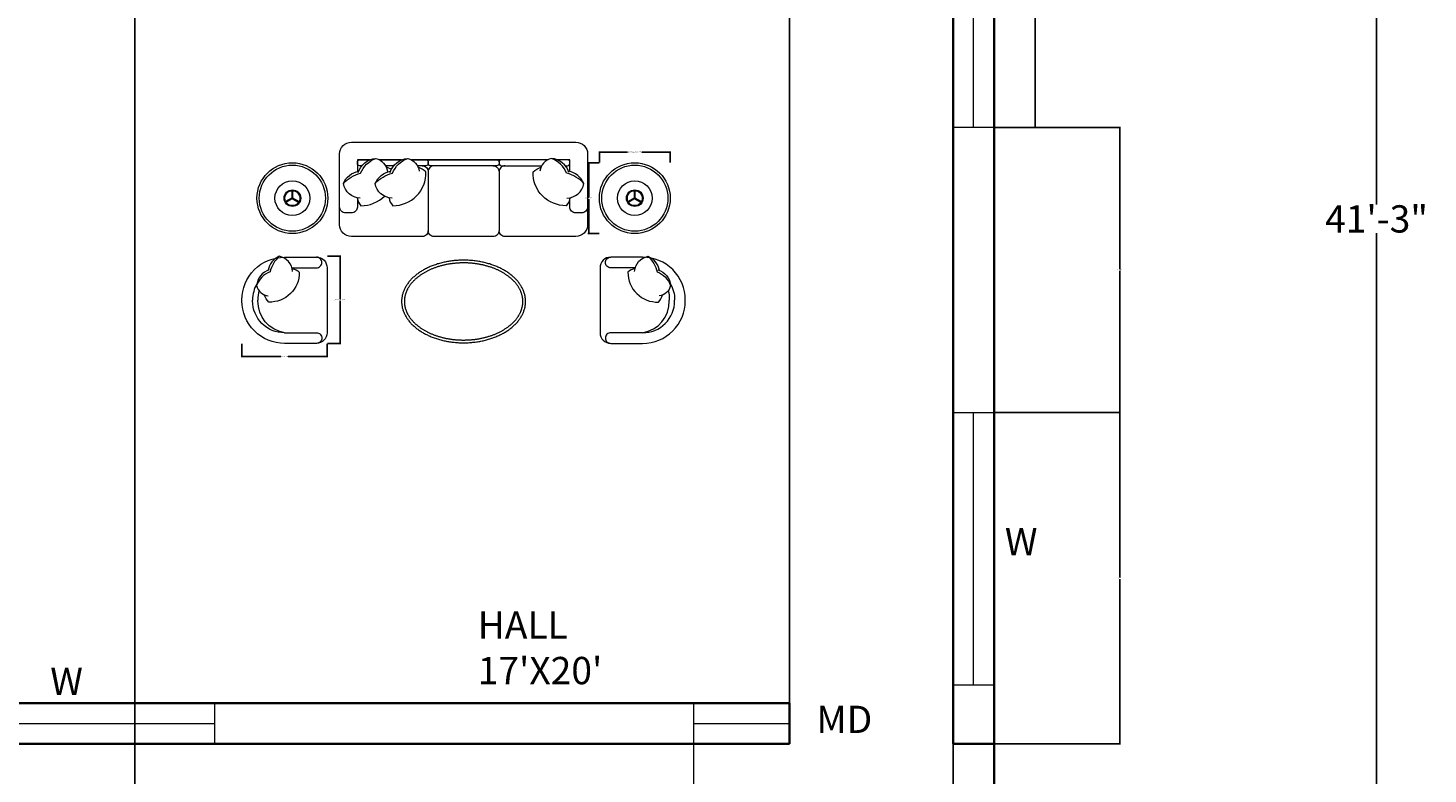
# Model space of a CAD drawing. Units: inches. Extents: x -4347 to -3836, y 955 to 1521.
# Tile 8 of 11: x -4144 to -3836, y 1120 to 1284. Entities that reach past the tile are written whole.
import ezdxf

# ---------------------------------------------------------------- set-up
doc = ezdxf.new("R2010")
doc.units = ezdxf.units.IN
doc.header["$MEASUREMENT"] = 0
for name, color, linetype, lineweight in [('A-ANNO-DIMS', 2, 'Continuous', 18), ('A-ANNO-TEXT', 7, 'Continuous', 18), ('A-AREA-IDEN', 7, 'Continuous', 18), ('A-FLOR-STRS', 7, 'Continuous', 18), ('A-FURN', 8, 'Continuous', 13), ('A-GLAZ', 4, 'Continuous', 18), ('A-WALL', 7, 'Continuous', 35)]:
    doc.layers.add(name, color=color, linetype=linetype, lineweight=lineweight)
doc.styles.get("Standard").update_dxf_attribs({"font": 'arial.ttf'})
doc.dimstyles.get("Standard").update_dxf_attribs({"dimtxt": 0.18, "dimasz": 0.18, "dimexe": 0.18, "dimexo": 0.0625, "dimgap": 0.09, "dimtad": 0, "dimtih": 1, "dimtoh": 1, "dimdec": 0, "dimzin": 0, "dimdsep": 46, "dimlunit": 3, "dimtxsty": 'Standard', "dimcen": 0.09, "dimadec": 0, "dimazin": 0, "dimtfac": 1, "dimtdec": 0, "dimtofl": 0, "dimtmove": 0, "dimatfit": 3, "dimfxl": 1, "dimtolj": 1, "dimtzin": 0, "dimarcsym": 0})

# ---------------------------------------------------------------- blocks, each defined once
blk = doc.blocks.new('*D2')
at = {"layer": 'A-ANNO-DIMS', "color": 0, "lineweight": -2, "transparency": 16777216}
for p, q in [((-3931.52, 1489.79), (-3847.29, 1489.79)), ((-3847.47, 1489.61), (-3847.47, 1245.44)), ((-3847.47, 994.97), (-3847.47, 1239.13)), ((-3931.52, 994.79), (-3847.29, 994.79))]:
    blk.add_line(p, q, dxfattribs=at)
at = {"layer": 'A-ANNO-DIMS', "color": 0, "transparency": 16777216}
for points in [[(-3847.5, 1489.61), (-3847.44, 1489.61), (-3847.47, 1489.79)], [(-3847.5, 994.97), (-3847.44, 994.97), (-3847.47, 994.79)]]:
    blk.add_solid(points, dxfattribs=at)
at = {"layer": 'Defpoints', "color": 0, "transparency": 16777216}
for p in [(-3931.58, 1489.79), (-3931.58, 994.79), (-3847.47, 994.79)]:
    blk.add_point(p, dxfattribs=at)
at = {"layer": 'A-ANNO-DIMS', "color": 0, "transparency": 16777216, "insert": (-3847.47, 1242.29), "char_height": 6, "attachment_point": 5}
blk.add_mtext('\\A1;41\'-3"', dxfattribs=at)
blk = doc.blocks.new('ARMCHAIR')
at = {"ltscale": 0.03}
blk.add_lwpolyline([(18.73, 9.48), (18.73, 2.34, -0.414214), (16.39, 0), (9.37, 0, -0.414214), (0, 9.37), (0, 9.48), (0, 9.6, -0.414214), (9.37, 18.97), (16.39, 18.97, -0.414214), (18.73, 16.62), (18.73, 9.48)], format="xyb", dxfattribs=at)
for points in [[(8.18, 19.16, 0.14773), (6.17, 15.73, 0.213343), (3.22, 12.72, 0.178662)], [(11.13, 15.8, 0.356772), (8.18, 19.16, 0.249542), (5.75, 16.12, -9.61688)], [(11.01, 16.62), (16.39, 16.62, 0.414214), (17.56, 17.79), (17.56, 17.79, 0.414214), (16.39, 18.97)], [(6.01, 16.21, 0.306663), (3.22, 12.72, 0.30633), (5.77, 10.43, -0.872847)], [(11.06, 16.39, -0.165541), (12.61, 15.67, -0.425989), (5.9, 9.09, -0.121523), (4.98, 10.65, 7.115464)], [(3.27, 13.09, 0.130591), (2.34, 9.6), (2.34, 9.48)], [(9.37, 2.34, -0.414214), (2.34, 9.37), (2.34, 9.48)], [(3.76, 11.6, 0.072384), (3.51, 9.6), (3.51, 9.48)], [(9.37, 2.34, -0.372719), (3.51, 9.37), (3.51, 9.48)], [(9.37, 2.34), (16.39, 2.34, -0.414214), (17.56, 1.17), (17.56, 1.17, -0.414214), (16.39, 0)]]:
    blk.add_lwpolyline(points, format="xyb")
blk = doc.blocks.new('END-TABLE-ROUND')
at = {"ltscale": 0.03}
for p, q in [((7.71, 7.79), (7.71, 9.62)), ((7.87, 7.79), (7.87, 9.62)), ((7.75, 7.86), (6.16, 6.95)), ((7.83, 7.72), (6.25, 6.8)), ((7.75, 7.72), (9.34, 6.8)), ((7.83, 7.86), (9.42, 6.95))]:
    blk.add_line(p, q, dxfattribs=at)
for radius in [7.79, 3.83, 1.83, 1.64]:
    blk.add_circle((7.79, 7.79), radius, dxfattribs=at)
blk.add_circle((7.79, 7.79), 7.27)
blk = doc.blocks.new('GLAZ-60IN')
for p, q in [((0, 9), (60, 9)), ((0, 0), (0, 9)), ((60, 9), (60, 0)), ((0, 4.5), (60, 4.5)), ((60, 0), (0, 0))]:
    blk.add_line(p, q)
blk = doc.blocks.new('*D20')
at = {"layer": 'A-ANNO-DIMS', "color": 0, "lineweight": -2, "transparency": 16777216}
for p, q in [((-4078.22, 1234.06), (-4075.23, 1234.06)), ((-4075.41, 1233.88), (-4075.41, 1224.66)), ((-4075.41, 1215.08), (-4075.41, 1224.3)), ((-4078.22, 1214.9), (-4075.23, 1214.9))]:
    blk.add_line(p, q, dxfattribs=at)
at = {"layer": 'A-ANNO-DIMS', "color": 0, "transparency": 16777216}
for points in [[(-4075.44, 1233.88), (-4075.38, 1233.88), (-4075.41, 1234.06)], [(-4075.44, 1215.08), (-4075.38, 1215.08), (-4075.41, 1214.9)]]:
    blk.add_solid(points, dxfattribs=at)
at = {"layer": 'Defpoints', "color": 0, "transparency": 16777216}
for p in [(-4078.28, 1234.06), (-4075.41, 1234.06), (-4078.28, 1214.9)]:
    blk.add_point(p, dxfattribs=at)
at = {"layer": 'A-ANNO-DIMS', "color": 0, "transparency": 16777216, "insert": (-4075.41, 1224.48), "char_height": 0.18, "attachment_point": 5}
blk.add_mtext('\\A1;ARMCHAIR 1\'-7" TYP.', dxfattribs=at)
blk = doc.blocks.new('*D21')
at = {"layer": 'A-ANNO-DIMS', "color": 0, "lineweight": -2, "transparency": 16777216}
for p, q in [((-4097.01, 1214.84), (-4097.01, 1211.85)), ((-4078.28, 1214.84), (-4078.28, 1211.85)), ((-4096.83, 1212.03), (-4088.49, 1212.03)), ((-4078.46, 1212.03), (-4086.81, 1212.03))]:
    blk.add_line(p, q, dxfattribs=at)
at = {"layer": 'A-ANNO-DIMS', "color": 0, "transparency": 16777216}
for points in [[(-4096.83, 1212.06), (-4096.83, 1212), (-4097.01, 1212.03)], [(-4078.46, 1212.06), (-4078.46, 1212), (-4078.28, 1212.03)]]:
    blk.add_solid(points, dxfattribs=at)
at = {"layer": 'Defpoints', "color": 0, "transparency": 16777216}
for p in [(-4097.01, 1214.9), (-4078.28, 1214.9), (-4078.28, 1212.03)]:
    blk.add_point(p, dxfattribs=at)
at = {"layer": 'A-ANNO-DIMS', "color": 0, "transparency": 16777216, "insert": (-4087.65, 1212.03), "char_height": 0.18, "attachment_point": 5}
blk.add_mtext('\\A1;1\'-6 1/2" TYP.', dxfattribs=at)
blk = doc.blocks.new('*D22')
at = {"layer": 'A-ANNO-DIMS', "color": 0, "lineweight": -2, "transparency": 16777216}
for p, q in [((-4018.4, 1254.7), (-4018.4, 1257.15)), ((-4018.22, 1256.97), (-4012.18, 1256.97)), ((-4003, 1256.97), (-4009.03, 1256.97)), ((-4002.82, 1254.7), (-4002.82, 1257.15))]:
    blk.add_line(p, q, dxfattribs=at)
at = {"layer": 'A-ANNO-DIMS', "color": 0, "transparency": 16777216}
for points in [[(-4018.22, 1257), (-4018.22, 1256.94), (-4018.4, 1256.97)], [(-4003, 1257), (-4003, 1256.94), (-4002.82, 1256.97)]]:
    blk.add_solid(points, dxfattribs=at)
at = {"layer": 'Defpoints', "color": 0, "transparency": 16777216}
for p in [(-4002.82, 1256.97), (-4018.4, 1254.64), (-4002.82, 1254.64)]:
    blk.add_point(p, dxfattribs=at)
at = {"layer": 'A-ANNO-DIMS', "color": 0, "transparency": 16777216, "insert": (-4010.61, 1256.97), "char_height": 0.18, "attachment_point": 5}
blk.add_mtext('\\A1;END TABLE 1\'-3 1/2" TYP.', dxfattribs=at)
blk = doc.blocks.new('*D23')
at = {"layer": 'A-ANNO-DIMS', "color": 0, "lineweight": -2, "transparency": 16777216}
for p, q in [((-4018.46, 1254.64), (-4020.91, 1254.64)), ((-4020.73, 1254.46), (-4020.73, 1247.03)), ((-4020.73, 1239.24), (-4020.73, 1246.66)), ((-4018.46, 1239.06), (-4020.91, 1239.06))]:
    blk.add_line(p, q, dxfattribs=at)
at = {"layer": 'A-ANNO-DIMS', "color": 0, "transparency": 16777216}
for points in [[(-4020.76, 1254.46), (-4020.7, 1254.46), (-4020.73, 1254.64)], [(-4020.76, 1239.24), (-4020.7, 1239.24), (-4020.73, 1239.06)]]:
    blk.add_solid(points, dxfattribs=at)
at = {"layer": 'Defpoints', "color": 0, "transparency": 16777216}
for p in [(-4020.73, 1254.64), (-4018.4, 1254.64), (-4018.4, 1239.06)]:
    blk.add_point(p, dxfattribs=at)
at = {"layer": 'A-ANNO-DIMS', "color": 0, "transparency": 16777216, "insert": (-4020.73, 1246.85), "char_height": 0.18, "attachment_point": 5}
blk.add_mtext('\\A1;1\'-3 1/2" TYP.', dxfattribs=at)
blk = doc.blocks.new('*D28')
at = {"layer": 'A-ANNO-DIMS', "color": 0, "lineweight": -2, "transparency": 16777216}
for p, q in [((-3931.52, 1322.43), (-3922.4, 1322.43)), ((-3922.58, 1322.25), (-3922.58, 1292.61)), ((-3922.58, 1262.61), (-3922.58, 1292.25)), ((-3931.52, 1262.43), (-3922.4, 1262.43))]:
    blk.add_line(p, q, dxfattribs=at)
at = {"layer": 'A-ANNO-DIMS', "color": 0, "transparency": 16777216}
for points in [[(-3922.61, 1322.25), (-3922.55, 1322.25), (-3922.58, 1322.43)], [(-3922.61, 1262.61), (-3922.55, 1262.61), (-3922.58, 1262.43)]]:
    blk.add_solid(points, dxfattribs=at)
at = {"layer": 'Defpoints', "color": 0, "transparency": 16777216}
for p in [(-3931.58, 1322.43), (-3922.58, 1322.43), (-3931.58, 1262.43)]:
    blk.add_point(p, dxfattribs=at)
at = {"layer": 'A-ANNO-DIMS', "color": 0, "transparency": 16777216, "insert": (-3922.58, 1292.43), "char_height": 0.18, "attachment_point": 5}
blk.add_mtext('\\A1;GLAZING 5\'-0" TYP.', dxfattribs=at)
blk = doc.blocks.new('*D44')
at = {"layer": 'A-ANNO-DIMS', "color": 0, "lineweight": -2, "transparency": 16777216}
for p, q in [((-3931.52, 1199.71), (-3903.75, 1199.71)), ((-3903.93, 1199.53), (-3903.93, 1163.43)), ((-3903.93, 1126.97), (-3903.93, 1163.07)), ((-3931.52, 1126.79), (-3903.75, 1126.79))]:
    blk.add_line(p, q, dxfattribs=at)
at = {"layer": 'A-ANNO-DIMS', "color": 0, "transparency": 16777216}
for points in [[(-3903.96, 1199.53), (-3903.9, 1199.53), (-3903.93, 1199.71)], [(-3903.96, 1126.97), (-3903.9, 1126.97), (-3903.93, 1126.79)]]:
    blk.add_solid(points, dxfattribs=at)
at = {"layer": 'Defpoints', "color": 0, "transparency": 16777216}
for p in [(-3931.58, 1199.71), (-3903.93, 1199.71), (-3931.58, 1126.79)]:
    blk.add_point(p, dxfattribs=at)
at = {"layer": 'A-ANNO-DIMS', "color": 0, "transparency": 16777216, "insert": (-3903.93, 1163.25), "char_height": 0.18, "attachment_point": 5}
blk.add_mtext('\\A1;6\'-1"', dxfattribs=at)
blk = doc.blocks.new('*D45')
at = {"layer": 'A-ANNO-DIMS', "color": 0, "lineweight": -2, "transparency": 16777216}
for p, q in [((-3931.52, 1262.43), (-3903.75, 1262.43)), ((-3903.93, 1262.25), (-3903.93, 1231.25)), ((-3903.93, 1199.89), (-3903.93, 1230.89)), ((-3931.52, 1199.71), (-3903.75, 1199.71))]:
    blk.add_line(p, q, dxfattribs=at)
at = {"layer": 'A-ANNO-DIMS', "color": 0, "transparency": 16777216}
for points in [[(-3903.96, 1262.25), (-3903.9, 1262.25), (-3903.93, 1262.43)], [(-3903.96, 1199.89), (-3903.9, 1199.89), (-3903.93, 1199.71)]]:
    blk.add_solid(points, dxfattribs=at)
at = {"layer": 'Defpoints', "color": 0, "transparency": 16777216}
for p in [(-3931.58, 1262.43), (-3903.93, 1262.43), (-3931.58, 1199.71)]:
    blk.add_point(p, dxfattribs=at)
at = {"layer": 'A-ANNO-DIMS', "color": 0, "transparency": 16777216, "insert": (-3903.93, 1231.07), "char_height": 0.18, "attachment_point": 5}
blk.add_mtext('\\A1;5\'-2 1/2"', dxfattribs=at)
blk = doc.blocks.new('*D47')
at = {"layer": 'A-ANNO-DIMS', "color": 0, "lineweight": -2, "transparency": 16777216}
for p, q in [((-4120.58, 1288.73), (-4120.58, 966.96)), ((-3940.58, 1288.73), (-3940.58, 966.96)), ((-4120.4, 967.14), (-4030.97, 967.14)), ((-3940.76, 967.14), (-4030.19, 967.14))]:
    blk.add_line(p, q, dxfattribs=at)
at = {"layer": 'A-ANNO-DIMS', "color": 0, "transparency": 16777216}
for points in [[(-4120.4, 967.17), (-4120.4, 967.11), (-4120.58, 967.14)], [(-3940.76, 967.17), (-3940.76, 967.11), (-3940.58, 967.14)]]:
    blk.add_solid(points, dxfattribs=at)
at = {"layer": 'Defpoints', "color": 0, "transparency": 16777216}
for p in [(-4120.58, 1288.79), (-3940.58, 1288.79), (-3940.58, 967.14)]:
    blk.add_point(p, dxfattribs=at)
at = {"layer": 'A-ANNO-DIMS', "color": 0, "transparency": 16777216, "insert": (-4030.58, 967.14), "char_height": 0.18, "attachment_point": 5}
blk.add_mtext('\\A1;15\'-0"', dxfattribs=at)
blk = doc.blocks.new('*D53')
at = {"layer": 'A-ANNO-DIMS', "color": 0, "lineweight": -2, "transparency": 16777216}
for p, q in [((-3976.58, 1135.85), (-3976.58, 1517.62)), ((-3976.4, 1517.44), (-3958.91, 1517.44)), ((-3940.76, 1517.44), (-3958.25, 1517.44)), ((-3940.58, 1135.85), (-3940.58, 1517.62))]:
    blk.add_line(p, q, dxfattribs=at)
at = {"layer": 'A-ANNO-DIMS', "color": 0, "transparency": 16777216}
for points in [[(-3976.4, 1517.47), (-3976.4, 1517.41), (-3976.58, 1517.44)], [(-3940.76, 1517.47), (-3940.76, 1517.41), (-3940.58, 1517.44)]]:
    blk.add_solid(points, dxfattribs=at)
at = {"layer": 'Defpoints', "color": 0, "transparency": 16777216}
for p in [(-3940.58, 1517.44), (-3976.58, 1135.79), (-3940.58, 1135.79)]:
    blk.add_point(p, dxfattribs=at)
at = {"layer": 'A-ANNO-DIMS', "color": 0, "transparency": 16777216, "insert": (-3958.58, 1517.44), "char_height": 0.18, "attachment_point": 5}
blk.add_mtext('\\A1;3\'-0"', dxfattribs=at)
blk = doc.blocks.new('*D54')
at = {"layer": 'A-ANNO-DIMS', "color": 0, "lineweight": -2, "transparency": 16777216}
for p, q in [((-3997.76, 1126.79), (-4346.41, 1126.79)), ((-4346.23, 1126.61), (-4346.23, 1111.97)), ((-4346.23, 1096.97), (-4346.23, 1111.61)), ((-3997.76, 1096.79), (-4346.41, 1096.79))]:
    blk.add_line(p, q, dxfattribs=at)
at = {"layer": 'A-ANNO-DIMS', "color": 0, "transparency": 16777216}
for points in [[(-4346.26, 1126.61), (-4346.2, 1126.61), (-4346.23, 1126.79)], [(-4346.26, 1096.97), (-4346.2, 1096.97), (-4346.23, 1096.79)]]:
    blk.add_solid(points, dxfattribs=at)
at = {"layer": 'Defpoints', "color": 0, "transparency": 16777216}
for p in [(-4346.23, 1126.79), (-3997.69, 1126.79), (-3997.69, 1096.79)]:
    blk.add_point(p, dxfattribs=at)
at = {"layer": 'A-ANNO-DIMS', "color": 0, "transparency": 16777216, "insert": (-4346.23, 1111.79), "char_height": 0.18, "attachment_point": 5}
blk.add_mtext('\\A1;2\'-6"', dxfattribs=at)

msp = doc.modelspace()

# ---------------------------------------------------------------- linework, layer by layer
at = {"layer": 'A-FLOR-STRS'}
msp.add_line((-3997.69, 1126.79), (-3997.69, 1116.79), dxfattribs=at)
at = {"layer": 'A-FURN', "ltscale": 0.03}
msp.add_lwpolyline([(-4020.99, 1241, -0.414214), (-4023.59, 1238.41), (-4039.17, 1238.41, -0.414214), (-4040.47, 1239.7, -0.414214), (-4041.77, 1238.41), (-4054.75, 1238.41, -0.414214), (-4056.05, 1239.7, -0.414214), (-4057.35, 1238.41), (-4072.93, 1238.41, -0.414214), (-4075.53, 1241), (-4075.53, 1256.58, -0.414214), (-4072.93, 1259.18), (-4023.59, 1259.18, -0.414214), (-4020.99, 1256.58)], format="xyb", close=True, dxfattribs=at)
at = {"layer": 'A-FURN'}
for points in [[(-4074.7, 1250.1, -0.14773), (-4070.91, 1252.34, -0.213343), (-4067.56, 1255.61, -0.178662)], [(-4068.9, 1255.29), (-4071.63, 1255.29), (-4071.63, 1252.73, -0.414214)], [(-4070.64, 1253.99), (-4071.11, 1253.99, -0.414214), (-4071.63, 1254.51), (-4071.63, 1254.77, -0.414214), (-4071.11, 1255.29)], [(-4071.43, 1252.51, -0.306663), (-4067.56, 1255.61, -0.30633), (-4065.03, 1252.78, 0.872847)], [(-4071.11, 1255.29), (-4068.9, 1255.29, -0.414214)], [(-4067.71, 1250.1, -0.14773), (-4063.91, 1252.34, -0.213343), (-4060.56, 1255.61, -0.178662)], [(-4066.74, 1255.29), (-4061.91, 1255.29, -0.414214)], [(-4063.65, 1253.99), (-4065.43, 1253.99, -0.414214)], [(-4064.18, 1253.15, 0.071865), (-4065.27, 1253.66, -7.115464)], [(-4064.64, 1246.91, 0.165541), (-4063.84, 1245.2, 0.425989), (-4056.55, 1252.63, 0.121523), (-4058.28, 1253.66, -7.115464)], [(-4064.44, 1252.51, -0.306663), (-4060.56, 1255.61, -0.30633), (-4058.03, 1252.78, 0.872847)], [(-4059.75, 1255.29), (-4056.57, 1255.29, -0.414214), (-4056.05, 1254.77), (-4056.05, 1254.51, -0.414214), (-4056.57, 1253.99), (-4058.44, 1253.99, -0.414214)], [(-4057.35, 1253.99, -0.414214), (-4056.05, 1252.69), (-4056.05, 1239.7, -0.414214)], [(-4054.75, 1253.99, 0.414214), (-4056.05, 1252.69)], [(-4041.77, 1253.99, -0.414214), (-4040.47, 1252.69)], [(-4029.78, 1255.29), (-4039.95, 1255.29, 0.414214), (-4040.47, 1254.77), (-4040.47, 1254.51, 0.414214), (-4039.95, 1253.99), (-4031.09, 1253.99, 0.414214)], [(-4039.17, 1253.99, 0.414214), (-4040.47, 1252.69), (-4040.47, 1239.7, 0.414214)], [(-4024.89, 1246.91, -0.165541), (-4025.69, 1245.2, -0.425989), (-4032.98, 1252.63, -0.121523), (-4031.25, 1253.66, 7.115464)], [(-4025.09, 1252.51, 0.306663), (-4028.96, 1255.61, 0.30633), (-4031.49, 1252.78, -0.872847)], [(-4021.82, 1250.1, 0.14773), (-4025.62, 1252.34, 0.213343), (-4028.96, 1255.61, 0.178662)], [(-4025.41, 1255.29), (-4027.62, 1255.29, 0.414214)], [(-4025.88, 1253.99), (-4025.41, 1253.99, 0.414214), (-4024.89, 1254.51), (-4024.89, 1254.77, 0.414214), (-4025.41, 1255.29)], [(-4070.98, 1246.83, -0.356772), (-4074.7, 1250.1, -0.249542), (-4071.33, 1252.8, 9.61688)], [(-4063.99, 1246.83, -0.356772), (-4067.71, 1250.1, -0.249542), (-4064.34, 1252.8, 9.61688)], [(-4025.54, 1246.83, 0.356772), (-4021.82, 1250.1, 0.249542), (-4025.19, 1252.8, -9.61688)], [(-4071.64, 1246.91, 0.165541), (-4070.83, 1245.2, 0.200231), (-4065.68, 1247.28, 0.121523)], [(-4071.63, 1246.91), (-4071.63, 1244.9, -0.414214), (-4072.93, 1243.6), (-4074.23, 1243.6, -0.414214), (-4075.53, 1244.9)], [(-4020.99, 1244.9, -0.414214), (-4022.29, 1243.6), (-4023.59, 1243.6, -0.414214), (-4024.89, 1244.9), (-4024.89, 1246.91)]]:
    msp.add_lwpolyline(points, format="xyb", dxfattribs=at)
for points in [[(-4061.91, 1255.29), (-4066.74, 1255.29)], [(-4029.78, 1255.29), (-4059.75, 1255.29)], [(-4024.89, 1252.73), (-4024.89, 1255.29), (-4027.62, 1255.29)]]:
    msp.add_lwpolyline(points, dxfattribs=at)
msp.add_lwpolyline([(-4055.53, 1255.29), (-4040.99, 1255.29, -0.414214), (-4040.47, 1254.77), (-4040.47, 1254.51, -0.414214), (-4040.99, 1253.99), (-4055.53, 1253.99, -0.414214), (-4056.05, 1254.51), (-4056.05, 1254.77, -0.414214)], format="xyb", close=True, dxfattribs=at)
at = {"layer": 'A-FURN', "ltscale": 0.03}
msp.add_polyline3d([(-4034.63, 1224.12, 0), (-4034.63, 1224.3, 0), (-4034.64, 1224.47, 0), (-4034.65, 1224.64, 0), (-4034.67, 1224.81, 0), (-4034.69, 1224.98, 0), (-4034.72, 1225.15, 0), (-4034.75, 1225.32, 0), (-4034.78, 1225.49, 0), (-4034.83, 1225.66, 0), (-4034.87, 1225.83, 0), (-4034.92, 1226, 0), (-4034.98, 1226.17, 0), (-4035.04, 1226.34, 0), (-4035.1, 1226.5, 0), (-4035.17, 1226.67, 0), (-4035.25, 1226.83, 0), (-4035.33, 1227, 0), (-4035.41, 1227.16, 0), (-4035.5, 1227.32, 0), (-4035.59, 1227.48, 0), (-4035.69, 1227.64, 0), (-4035.79, 1227.8, 0), (-4035.9, 1227.96, 0), (-4036.01, 1228.11, 0), (-4036.13, 1228.27, 0), (-4036.25, 1228.42, 0), (-4036.37, 1228.57, 0), (-4036.5, 1228.72, 0), (-4036.63, 1228.87, 0), (-4036.77, 1229.01, 0), (-4036.91, 1229.16, 0), (-4037.05, 1229.3, 0), (-4037.2, 1229.44, 0), (-4037.35, 1229.58, 0), (-4037.51, 1229.71, 0), (-4037.67, 1229.85, 0), (-4037.84, 1229.98, 0), (-4038, 1230.11, 0), (-4038.18, 1230.24, 0), (-4038.35, 1230.37, 0), (-4038.53, 1230.49, 0), (-4038.71, 1230.61, 0), (-4038.9, 1230.73, 0), (-4039.09, 1230.85, 0), (-4039.28, 1230.96, 0), (-4039.48, 1231.07, 0), (-4039.67, 1231.18, 0), (-4039.88, 1231.29, 0), (-4040.08, 1231.4, 0), (-4040.29, 1231.5, 0), (-4040.5, 1231.6, 0), (-4040.71, 1231.69, 0), (-4040.93, 1231.79, 0), (-4041.15, 1231.88, 0), (-4041.37, 1231.97, 0), (-4041.59, 1232.05, 0), (-4041.82, 1232.13, 0), (-4042.05, 1232.21, 0), (-4042.28, 1232.29, 0), (-4042.51, 1232.37, 0), (-4042.75, 1232.44, 0), (-4042.98, 1232.5, 0), (-4043.22, 1232.57, 0), (-4043.46, 1232.63, 0), (-4043.71, 1232.69, 0), (-4043.95, 1232.75, 0), (-4044.2, 1232.8, 0), (-4044.44, 1232.85, 0), (-4044.69, 1232.9, 0), (-4044.94, 1232.94, 0), (-4045.19, 1232.98, 0), (-4045.44, 1233.02, 0), (-4045.7, 1233.05, 0), (-4045.95, 1233.08, 0), (-4046.21, 1233.11, 0), (-4046.46, 1233.13, 0), (-4046.72, 1233.15, 0), (-4046.97, 1233.17, 0), (-4047.23, 1233.19, 0), (-4047.49, 1233.2, 0), (-4047.75, 1233.21, 0), (-4048, 1233.21, 0), (-4048.26, 1233.21, 0), (-4048.52, 1233.21, 0), (-4048.78, 1233.21, 0), (-4049.04, 1233.2, 0), (-4049.29, 1233.19, 0), (-4049.55, 1233.17, 0), (-4049.81, 1233.15, 0), (-4050.06, 1233.13, 0), (-4050.32, 1233.11, 0), (-4050.57, 1233.08, 0), (-4050.83, 1233.05, 0), (-4051.08, 1233.02, 0), (-4051.33, 1232.98, 0), (-4051.58, 1232.94, 0), (-4051.83, 1232.9, 0), (-4052.08, 1232.85, 0), (-4052.33, 1232.8, 0), (-4052.57, 1232.75, 0), (-4052.82, 1232.69, 0), (-4053.06, 1232.63, 0), (-4053.3, 1232.57, 0), (-4053.54, 1232.5, 0), (-4053.78, 1232.44, 0), (-4054.01, 1232.37, 0), (-4054.24, 1232.29, 0), (-4054.47, 1232.21, 0), (-4054.7, 1232.13, 0), (-4054.93, 1232.05, 0), (-4055.15, 1231.97, 0), (-4055.37, 1231.88, 0), (-4055.59, 1231.79, 0), (-4055.81, 1231.69, 0), (-4056.02, 1231.6, 0), (-4056.23, 1231.5, 0), (-4056.44, 1231.4, 0), (-4056.65, 1231.29, 0), (-4056.85, 1231.18, 0), (-4057.05, 1231.07, 0), (-4057.24, 1230.96, 0), (-4057.43, 1230.85, 0), (-4057.62, 1230.73, 0), (-4057.81, 1230.61, 0), (-4057.99, 1230.49, 0), (-4058.17, 1230.37, 0), (-4058.35, 1230.24, 0), (-4058.52, 1230.11, 0), (-4058.69, 1229.98, 0), (-4058.85, 1229.85, 0), (-4059.01, 1229.71, 0), (-4059.17, 1229.58, 0), (-4059.32, 1229.44, 0), (-4059.47, 1229.3, 0), (-4059.62, 1229.16, 0), (-4059.76, 1229.01, 0), (-4059.89, 1228.87, 0), (-4060.03, 1228.72, 0), (-4060.15, 1228.57, 0), (-4060.28, 1228.42, 0), (-4060.4, 1228.27, 0), (-4060.51, 1228.11, 0), (-4060.62, 1227.96, 0), (-4060.73, 1227.8, 0), (-4060.83, 1227.64, 0), (-4060.93, 1227.48, 0), (-4061.02, 1227.32, 0), (-4061.11, 1227.16, 0), (-4061.2, 1227, 0), (-4061.27, 1226.83, 0), (-4061.35, 1226.67, 0), (-4061.42, 1226.5, 0), (-4061.48, 1226.34, 0), (-4061.54, 1226.17, 0), (-4061.6, 1226, 0), (-4061.65, 1225.83, 0), (-4061.7, 1225.66, 0), (-4061.74, 1225.49, 0), (-4061.78, 1225.32, 0), (-4061.81, 1225.15, 0), (-4061.83, 1224.98, 0), (-4061.86, 1224.81, 0), (-4061.87, 1224.64, 0), (-4061.89, 1224.47, 0), (-4061.89, 1224.3, 0), (-4061.89, 1224.12, 0), (-4061.89, 1223.95, 0), (-4061.89, 1223.78, 0), (-4061.87, 1223.61, 0), (-4061.86, 1223.44, 0), (-4061.83, 1223.26, 0), (-4061.81, 1223.09, 0), (-4061.78, 1222.92, 0), (-4061.74, 1222.75, 0), (-4061.7, 1222.58, 0), (-4061.65, 1222.41, 0), (-4061.6, 1222.25, 0), (-4061.54, 1222.08, 0), (-4061.48, 1221.91, 0), (-4061.42, 1221.74, 0), (-4061.35, 1221.58, 0), (-4061.27, 1221.41, 0), (-4061.2, 1221.25, 0), (-4061.11, 1221.09, 0), (-4061.02, 1220.93, 0), (-4060.93, 1220.76, 0), (-4060.83, 1220.61, 0), (-4060.73, 1220.45, 0), (-4060.62, 1220.29, 0), (-4060.51, 1220.14, 0), (-4060.4, 1219.98, 0), (-4060.28, 1219.83, 0), (-4060.15, 1219.68, 0), (-4060.03, 1219.53, 0), (-4059.89, 1219.38, 0), (-4059.76, 1219.24, 0), (-4059.62, 1219.09, 0), (-4059.47, 1218.95, 0), (-4059.32, 1218.81, 0), (-4059.17, 1218.67, 0), (-4059.01, 1218.53, 0), (-4058.85, 1218.4, 0), (-4058.69, 1218.27, 0), (-4058.52, 1218.14, 0), (-4058.35, 1218.01, 0), (-4058.17, 1217.88, 0), (-4057.99, 1217.76, 0), (-4057.81, 1217.64, 0), (-4057.62, 1217.52, 0), (-4057.43, 1217.4, 0), (-4057.24, 1217.29, 0), (-4057.05, 1217.17, 0), (-4056.85, 1217.06, 0), (-4056.65, 1216.96, 0), (-4056.44, 1216.85, 0), (-4056.23, 1216.75, 0), (-4056.02, 1216.65, 0), (-4055.81, 1216.55, 0), (-4055.59, 1216.46, 0), (-4055.37, 1216.37, 0), (-4055.15, 1216.28, 0), (-4054.93, 1216.2, 0), (-4054.7, 1216.11, 0), (-4054.47, 1216.03, 0), (-4054.24, 1215.96, 0), (-4054.01, 1215.88, 0), (-4053.78, 1215.81, 0), (-4053.54, 1215.74, 0), (-4053.3, 1215.68, 0), (-4053.06, 1215.62, 0), (-4052.82, 1215.56, 0), (-4052.57, 1215.5, 0), (-4052.33, 1215.45, 0), (-4052.08, 1215.4, 0), (-4051.83, 1215.35, 0), (-4051.58, 1215.31, 0), (-4051.33, 1215.27, 0), (-4051.08, 1215.23, 0), (-4050.83, 1215.2, 0), (-4050.57, 1215.17, 0), (-4050.32, 1215.14, 0), (-4050.06, 1215.11, 0), (-4049.81, 1215.09, 0), (-4049.55, 1215.08, 0), (-4049.29, 1215.06, 0), (-4049.04, 1215.05, 0), (-4048.78, 1215.04, 0), (-4048.52, 1215.04, 0), (-4048.26, 1215.03, 0), (-4048, 1215.04, 0), (-4047.75, 1215.04, 0), (-4047.49, 1215.05, 0), (-4047.23, 1215.06, 0), (-4046.97, 1215.08, 0), (-4046.72, 1215.09, 0), (-4046.46, 1215.11, 0), (-4046.21, 1215.14, 0), (-4045.95, 1215.17, 0), (-4045.7, 1215.2, 0), (-4045.44, 1215.23, 0), (-4045.19, 1215.27, 0), (-4044.94, 1215.31, 0), (-4044.69, 1215.35, 0), (-4044.44, 1215.4, 0), (-4044.2, 1215.45, 0), (-4043.95, 1215.5, 0), (-4043.71, 1215.56, 0), (-4043.46, 1215.62, 0), (-4043.22, 1215.68, 0), (-4042.98, 1215.74, 0), (-4042.75, 1215.81, 0), (-4042.51, 1215.88, 0), (-4042.28, 1215.96, 0), (-4042.05, 1216.03, 0), (-4041.82, 1216.11, 0), (-4041.59, 1216.2, 0), (-4041.37, 1216.28, 0), (-4041.15, 1216.37, 0), (-4040.93, 1216.46, 0), (-4040.71, 1216.55, 0), (-4040.5, 1216.65, 0), (-4040.29, 1216.75, 0), (-4040.08, 1216.85, 0), (-4039.88, 1216.96, 0), (-4039.67, 1217.06, 0), (-4039.48, 1217.17, 0), (-4039.28, 1217.29, 0), (-4039.09, 1217.4, 0), (-4038.9, 1217.52, 0), (-4038.71, 1217.64, 0), (-4038.53, 1217.76, 0), (-4038.35, 1217.88, 0), (-4038.18, 1218.01, 0), (-4038, 1218.14, 0), (-4037.84, 1218.27, 0), (-4037.67, 1218.4, 0), (-4037.51, 1218.53, 0), (-4037.35, 1218.67, 0), (-4037.2, 1218.81, 0), (-4037.05, 1218.95, 0), (-4036.91, 1219.09, 0), (-4036.77, 1219.24, 0), (-4036.63, 1219.38, 0), (-4036.5, 1219.53, 0), (-4036.37, 1219.68, 0), (-4036.25, 1219.83, 0), (-4036.13, 1219.98, 0), (-4036.01, 1220.14, 0), (-4035.9, 1220.29, 0), (-4035.79, 1220.45, 0), (-4035.69, 1220.61, 0), (-4035.59, 1220.76, 0), (-4035.5, 1220.93, 0), (-4035.41, 1221.09, 0), (-4035.33, 1221.25, 0), (-4035.25, 1221.41, 0), (-4035.17, 1221.58, 0), (-4035.1, 1221.74, 0), (-4035.04, 1221.91, 0), (-4034.98, 1222.08, 0), (-4034.92, 1222.25, 0), (-4034.87, 1222.41, 0), (-4034.83, 1222.58, 0), (-4034.78, 1222.75, 0), (-4034.75, 1222.92, 0), (-4034.72, 1223.09, 0), (-4034.69, 1223.26, 0), (-4034.67, 1223.44, 0), (-4034.65, 1223.61, 0), (-4034.64, 1223.78, 0), (-4034.63, 1223.95, 0), (-4034.63, 1224.12, 0)], dxfattribs=at)
at = {"layer": 'A-FURN'}
msp.add_polyline3d([(-4035.23, 1224.12, 0), (-4035.23, 1224.22, 0), (-4035.24, 1224.31, 0), (-4035.24, 1224.4, 0), (-4035.25, 1224.5, 0), (-4035.25, 1224.59, 0), (-4035.26, 1224.69, 0), (-4035.27, 1224.78, 0), (-4035.29, 1224.88, 0), (-4035.3, 1224.97, 0), (-4035.32, 1225.07, 0), (-4035.33, 1225.17, 0), (-4035.35, 1225.26, 0), (-4035.38, 1225.36, 0), (-4035.4, 1225.46, 0), (-4035.42, 1225.56, 0), (-4035.45, 1225.66, 0), (-4035.48, 1225.75, 0), (-4035.51, 1225.85, 0), (-4035.54, 1225.95, 0), (-4035.58, 1226.05, 0), (-4035.61, 1226.15, 0), (-4035.65, 1226.25, 0), (-4035.69, 1226.35, 0), (-4035.74, 1226.45, 0), (-4035.78, 1226.55, 0), (-4035.83, 1226.65, 0), (-4035.88, 1226.75, 0), (-4035.93, 1226.84, 0), (-4035.98, 1226.94, 0), (-4036.04, 1227.04, 0), (-4036.1, 1227.14, 0), (-4036.16, 1227.24, 0), (-4036.22, 1227.34, 0), (-4036.28, 1227.44, 0), (-4036.35, 1227.54, 0), (-4036.42, 1227.64, 0), (-4036.49, 1227.73, 0), (-4036.56, 1227.83, 0), (-4036.63, 1227.93, 0), (-4036.71, 1228.03, 0), (-4036.79, 1228.12, 0), (-4036.87, 1228.22, 0), (-4036.95, 1228.31, 0), (-4037.03, 1228.41, 0), (-4037.12, 1228.5, 0), (-4037.21, 1228.6, 0), (-4037.3, 1228.69, 0), (-4037.4, 1228.78, 0), (-4037.49, 1228.88, 0), (-4037.59, 1228.97, 0), (-4037.69, 1229.06, 0), (-4037.79, 1229.15, 0), (-4037.9, 1229.24, 0), (-4038, 1229.33, 0), (-4038.11, 1229.42, 0), (-4038.22, 1229.5, 0), (-4038.33, 1229.59, 0), (-4038.45, 1229.68, 0), (-4038.56, 1229.76, 0), (-4038.68, 1229.84, 0), (-4038.8, 1229.93, 0), (-4038.92, 1230.01, 0), (-4039.04, 1230.09, 0), (-4039.16, 1230.17, 0), (-4039.29, 1230.25, 0), (-4039.42, 1230.33, 0), (-4039.54, 1230.41, 0), (-4039.67, 1230.48, 0), (-4039.81, 1230.56, 0), (-4039.94, 1230.63, 0), (-4040.07, 1230.7, 0), (-4040.21, 1230.77, 0), (-4040.34, 1230.84, 0), (-4040.48, 1230.91, 0), (-4040.62, 1230.98, 0), (-4040.76, 1231.05, 0), (-4040.91, 1231.11, 0), (-4041.05, 1231.18, 0), (-4041.19, 1231.24, 0), (-4041.34, 1231.3, 0), (-4041.49, 1231.36, 0), (-4041.63, 1231.42, 0), (-4041.78, 1231.47, 0), (-4041.93, 1231.53, 0), (-4042.08, 1231.58, 0), (-4042.23, 1231.64, 0), (-4042.38, 1231.69, 0), (-4042.53, 1231.74, 0), (-4042.68, 1231.78, 0), (-4042.84, 1231.83, 0), (-4042.99, 1231.88, 0), (-4043.14, 1231.92, 0), (-4043.29, 1231.96, 0), (-4043.45, 1232, 0), (-4043.6, 1232.04, 0), (-4043.75, 1232.08, 0), (-4043.91, 1232.12, 0), (-4044.06, 1232.15, 0), (-4044.22, 1232.19, 0), (-4044.37, 1232.22, 0), (-4044.53, 1232.25, 0), (-4044.68, 1232.28, 0), (-4044.84, 1232.31, 0), (-4044.99, 1232.34, 0), (-4045.15, 1232.36, 0), (-4045.31, 1232.39, 0), (-4045.46, 1232.41, 0), (-4045.62, 1232.43, 0), (-4045.78, 1232.45, 0), (-4045.93, 1232.47, 0), (-4046.09, 1232.49, 0), (-4046.25, 1232.51, 0), (-4046.41, 1232.52, 0), (-4046.56, 1232.54, 0), (-4046.72, 1232.55, 0), (-4046.88, 1232.56, 0), (-4047.04, 1232.57, 0), (-4047.19, 1232.58, 0), (-4047.35, 1232.59, 0), (-4047.51, 1232.59, 0), (-4047.67, 1232.6, 0), (-4047.83, 1232.6, 0), (-4047.98, 1232.6, 0), (-4048.14, 1232.61, 0), (-4048.3, 1232.61, 0), (-4048.46, 1232.61, 0), (-4048.62, 1232.6, 0), (-4048.78, 1232.6, 0), (-4048.93, 1232.6, 0), (-4049.09, 1232.59, 0), (-4049.25, 1232.58, 0), (-4049.41, 1232.57, 0), (-4049.57, 1232.56, 0), (-4049.72, 1232.55, 0), (-4049.88, 1232.54, 0), (-4050.04, 1232.53, 0), (-4050.2, 1232.51, 0), (-4050.35, 1232.5, 0), (-4050.51, 1232.48, 0), (-4050.67, 1232.46, 0), (-4050.82, 1232.44, 0), (-4050.98, 1232.42, 0), (-4051.14, 1232.4, 0), (-4051.29, 1232.37, 0), (-4051.45, 1232.35, 0), (-4051.61, 1232.32, 0), (-4051.76, 1232.3, 0), (-4051.92, 1232.27, 0), (-4052.07, 1232.24, 0), (-4052.23, 1232.2, 0), (-4052.38, 1232.17, 0), (-4052.54, 1232.14, 0), (-4052.69, 1232.1, 0), (-4052.85, 1232.06, 0), (-4053, 1232.02, 0), (-4053.15, 1231.98, 0), (-4053.31, 1231.94, 0), (-4053.46, 1231.9, 0), (-4053.61, 1231.85, 0), (-4053.76, 1231.81, 0), (-4053.91, 1231.76, 0), (-4054.07, 1231.71, 0), (-4054.22, 1231.66, 0), (-4054.37, 1231.61, 0), (-4054.52, 1231.56, 0), (-4054.67, 1231.5, 0), (-4054.82, 1231.45, 0), (-4054.96, 1231.39, 0), (-4055.11, 1231.33, 0), (-4055.26, 1231.27, 0), (-4055.4, 1231.21, 0), (-4055.55, 1231.14, 0), (-4055.69, 1231.08, 0), (-4055.83, 1231.01, 0), (-4055.97, 1230.95, 0), (-4056.11, 1230.88, 0), (-4056.25, 1230.81, 0), (-4056.38, 1230.74, 0), (-4056.52, 1230.67, 0), (-4056.65, 1230.59, 0), (-4056.78, 1230.52, 0), (-4056.91, 1230.44, 0), (-4057.04, 1230.37, 0), (-4057.17, 1230.29, 0), (-4057.3, 1230.21, 0), (-4057.42, 1230.13, 0), (-4057.54, 1230.05, 0), (-4057.67, 1229.97, 0), (-4057.79, 1229.89, 0), (-4057.9, 1229.8, 0), (-4058.02, 1229.72, 0), (-4058.13, 1229.63, 0), (-4058.25, 1229.55, 0), (-4058.36, 1229.46, 0), (-4058.47, 1229.37, 0), (-4058.57, 1229.28, 0), (-4058.68, 1229.19, 0), (-4058.78, 1229.1, 0), (-4058.88, 1229.01, 0), (-4058.98, 1228.92, 0), (-4059.08, 1228.83, 0), (-4059.17, 1228.74, 0), (-4059.27, 1228.64, 0), (-4059.36, 1228.55, 0), (-4059.44, 1228.46, 0), (-4059.53, 1228.36, 0), (-4059.61, 1228.27, 0), (-4059.7, 1228.17, 0), (-4059.78, 1228.07, 0), (-4059.85, 1227.98, 0), (-4059.93, 1227.88, 0), (-4060, 1227.78, 0), (-4060.07, 1227.69, 0), (-4060.14, 1227.59, 0), (-4060.21, 1227.49, 0), (-4060.27, 1227.39, 0), (-4060.34, 1227.29, 0), (-4060.4, 1227.19, 0), (-4060.46, 1227.09, 0), (-4060.51, 1226.99, 0), (-4060.57, 1226.89, 0), (-4060.62, 1226.79, 0), (-4060.67, 1226.7, 0), (-4060.72, 1226.6, 0), (-4060.76, 1226.5, 0), (-4060.81, 1226.4, 0), (-4060.85, 1226.3, 0), (-4060.89, 1226.2, 0), (-4060.93, 1226.1, 0), (-4060.96, 1226, 0), (-4061, 1225.9, 0), (-4061.03, 1225.8, 0), (-4061.06, 1225.7, 0), (-4061.09, 1225.61, 0), (-4061.11, 1225.51, 0), (-4061.14, 1225.41, 0), (-4061.16, 1225.31, 0), (-4061.18, 1225.22, 0), (-4061.2, 1225.12, 0), (-4061.21, 1225.02, 0), (-4061.23, 1224.93, 0), (-4061.24, 1224.83, 0), (-4061.25, 1224.74, 0), (-4061.26, 1224.64, 0), (-4061.27, 1224.55, 0), (-4061.28, 1224.45, 0), (-4061.28, 1224.36, 0), (-4061.29, 1224.26, 0), (-4061.29, 1224.17, 0), (-4061.29, 1224.08, 0), (-4061.29, 1223.98, 0), (-4061.28, 1223.89, 0), (-4061.28, 1223.8, 0), (-4061.27, 1223.7, 0), (-4061.26, 1223.61, 0), (-4061.25, 1223.51, 0), (-4061.24, 1223.42, 0), (-4061.23, 1223.32, 0), (-4061.21, 1223.22, 0), (-4061.2, 1223.13, 0), (-4061.18, 1223.03, 0), (-4061.16, 1222.93, 0), (-4061.14, 1222.84, 0), (-4061.11, 1222.74, 0), (-4061.09, 1222.64, 0), (-4061.06, 1222.54, 0), (-4061.03, 1222.44, 0), (-4061, 1222.35, 0), (-4060.96, 1222.25, 0), (-4060.93, 1222.15, 0), (-4060.89, 1222.05, 0), (-4060.85, 1221.95, 0), (-4060.81, 1221.85, 0), (-4060.76, 1221.75, 0), (-4060.72, 1221.65, 0), (-4060.67, 1221.55, 0), (-4060.62, 1221.45, 0), (-4060.57, 1221.35, 0), (-4060.51, 1221.25, 0), (-4060.46, 1221.15, 0), (-4060.4, 1221.06, 0), (-4060.34, 1220.96, 0), (-4060.27, 1220.86, 0), (-4060.21, 1220.76, 0), (-4060.14, 1220.66, 0), (-4060.07, 1220.56, 0), (-4060, 1220.46, 0), (-4059.93, 1220.37, 0), (-4059.85, 1220.27, 0), (-4059.78, 1220.17, 0), (-4059.7, 1220.08, 0), (-4059.61, 1219.98, 0), (-4059.53, 1219.89, 0), (-4059.44, 1219.79, 0), (-4059.36, 1219.7, 0), (-4059.27, 1219.6, 0), (-4059.17, 1219.51, 0), (-4059.08, 1219.42, 0), (-4058.98, 1219.32, 0), (-4058.88, 1219.23, 0), (-4058.78, 1219.14, 0), (-4058.68, 1219.05, 0), (-4058.57, 1218.96, 0), (-4058.47, 1218.88, 0), (-4058.36, 1218.79, 0), (-4058.25, 1218.7, 0), (-4058.13, 1218.61, 0), (-4058.02, 1218.53, 0), (-4057.9, 1218.44, 0), (-4057.79, 1218.36, 0), (-4057.67, 1218.28, 0), (-4057.54, 1218.2, 0), (-4057.42, 1218.12, 0), (-4057.3, 1218.04, 0), (-4057.17, 1217.96, 0), (-4057.04, 1217.88, 0), (-4056.91, 1217.8, 0), (-4056.78, 1217.73, 0), (-4056.65, 1217.65, 0), (-4056.52, 1217.58, 0), (-4056.38, 1217.51, 0), (-4056.25, 1217.44, 0), (-4056.11, 1217.37, 0), (-4055.97, 1217.3, 0), (-4055.83, 1217.23, 0), (-4055.69, 1217.17, 0), (-4055.55, 1217.1, 0), (-4055.4, 1217.04, 0), (-4055.26, 1216.98, 0), (-4055.11, 1216.92, 0), (-4054.96, 1216.86, 0), (-4054.82, 1216.8, 0), (-4054.67, 1216.74, 0), (-4054.52, 1216.69, 0), (-4054.37, 1216.64, 0), (-4054.22, 1216.59, 0), (-4054.07, 1216.54, 0), (-4053.91, 1216.49, 0), (-4053.76, 1216.44, 0), (-4053.61, 1216.39, 0), (-4053.46, 1216.35, 0), (-4053.31, 1216.31, 0), (-4053.15, 1216.26, 0), (-4053, 1216.22, 0), (-4052.85, 1216.19, 0), (-4052.69, 1216.15, 0), (-4052.54, 1216.11, 0), (-4052.38, 1216.08, 0), (-4052.23, 1216.04, 0), (-4052.07, 1216.01, 0), (-4051.92, 1215.98, 0), (-4051.76, 1215.95, 0), (-4051.61, 1215.92, 0), (-4051.45, 1215.9, 0), (-4051.29, 1215.87, 0), (-4051.14, 1215.85, 0), (-4050.98, 1215.83, 0), (-4050.82, 1215.81, 0), (-4050.67, 1215.79, 0), (-4050.51, 1215.77, 0), (-4050.35, 1215.75, 0), (-4050.2, 1215.73, 0), (-4050.04, 1215.72, 0), (-4049.88, 1215.71, 0), (-4049.72, 1215.69, 0), (-4049.57, 1215.68, 0), (-4049.41, 1215.67, 0), (-4049.25, 1215.66, 0), (-4049.09, 1215.66, 0), (-4048.93, 1215.65, 0), (-4048.78, 1215.65, 0), (-4048.62, 1215.64, 0), (-4048.46, 1215.64, 0), (-4048.3, 1215.64, 0), (-4048.14, 1215.64, 0), (-4047.98, 1215.64, 0), (-4047.83, 1215.65, 0), (-4047.67, 1215.65, 0), (-4047.51, 1215.65, 0), (-4047.35, 1215.66, 0), (-4047.19, 1215.67, 0), (-4047.04, 1215.68, 0), (-4046.88, 1215.69, 0), (-4046.72, 1215.7, 0), (-4046.56, 1215.71, 0), (-4046.41, 1215.73, 0), (-4046.25, 1215.74, 0), (-4046.09, 1215.76, 0), (-4045.93, 1215.78, 0), (-4045.78, 1215.79, 0), (-4045.62, 1215.82, 0), (-4045.46, 1215.84, 0), (-4045.31, 1215.86, 0), (-4045.15, 1215.88, 0), (-4044.99, 1215.91, 0), (-4044.84, 1215.94, 0), (-4044.68, 1215.97, 0), (-4044.53, 1216, 0), (-4044.37, 1216.03, 0), (-4044.22, 1216.06, 0), (-4044.06, 1216.09, 0), (-4043.91, 1216.13, 0), (-4043.75, 1216.17, 0), (-4043.6, 1216.2, 0), (-4043.45, 1216.24, 0), (-4043.29, 1216.28, 0), (-4043.14, 1216.33, 0), (-4042.99, 1216.37, 0), (-4042.84, 1216.42, 0), (-4042.68, 1216.46, 0), (-4042.53, 1216.51, 0), (-4042.38, 1216.56, 0), (-4042.23, 1216.61, 0), (-4042.08, 1216.66, 0), (-4041.93, 1216.72, 0), (-4041.78, 1216.77, 0), (-4041.63, 1216.83, 0), (-4041.49, 1216.89, 0), (-4041.34, 1216.95, 0), (-4041.19, 1217.01, 0), (-4041.05, 1217.07, 0), (-4040.91, 1217.13, 0), (-4040.76, 1217.2, 0), (-4040.62, 1217.27, 0), (-4040.48, 1217.33, 0), (-4040.34, 1217.4, 0), (-4040.21, 1217.47, 0), (-4040.07, 1217.54, 0), (-4039.94, 1217.62, 0), (-4039.81, 1217.69, 0), (-4039.67, 1217.77, 0), (-4039.54, 1217.84, 0), (-4039.42, 1217.92, 0), (-4039.29, 1218, 0), (-4039.16, 1218.08, 0), (-4039.04, 1218.16, 0), (-4038.92, 1218.24, 0), (-4038.8, 1218.32, 0), (-4038.68, 1218.4, 0), (-4038.56, 1218.49, 0), (-4038.45, 1218.57, 0), (-4038.33, 1218.66, 0), (-4038.22, 1218.74, 0), (-4038.11, 1218.83, 0), (-4038, 1218.92, 0), (-4037.9, 1219.01, 0), (-4037.79, 1219.1, 0), (-4037.69, 1219.19, 0), (-4037.59, 1219.28, 0), (-4037.49, 1219.37, 0), (-4037.4, 1219.46, 0), (-4037.3, 1219.56, 0), (-4037.21, 1219.65, 0), (-4037.12, 1219.74, 0), (-4037.03, 1219.84, 0), (-4036.95, 1219.93, 0), (-4036.87, 1220.03, 0), (-4036.79, 1220.12, 0), (-4036.71, 1220.22, 0), (-4036.63, 1220.32, 0), (-4036.56, 1220.42, 0), (-4036.49, 1220.51, 0), (-4036.42, 1220.61, 0), (-4036.35, 1220.71, 0), (-4036.28, 1220.81, 0), (-4036.22, 1220.91, 0), (-4036.16, 1221.01, 0), (-4036.1, 1221.1, 0), (-4036.04, 1221.2, 0), (-4035.98, 1221.3, 0), (-4035.93, 1221.4, 0), (-4035.88, 1221.5, 0), (-4035.83, 1221.6, 0), (-4035.78, 1221.7, 0), (-4035.74, 1221.8, 0), (-4035.69, 1221.9, 0), (-4035.65, 1222, 0), (-4035.61, 1222.1, 0), (-4035.58, 1222.2, 0), (-4035.54, 1222.3, 0), (-4035.51, 1222.4, 0), (-4035.48, 1222.49, 0), (-4035.45, 1222.59, 0), (-4035.42, 1222.69, 0), (-4035.4, 1222.79, 0), (-4035.38, 1222.89, 0), (-4035.35, 1222.98, 0), (-4035.33, 1223.08, 0), (-4035.32, 1223.18, 0), (-4035.3, 1223.27, 0), (-4035.29, 1223.37, 0), (-4035.27, 1223.46, 0), (-4035.26, 1223.56, 0), (-4035.25, 1223.65, 0), (-4035.25, 1223.75, 0), (-4035.24, 1223.84, 0), (-4035.24, 1223.94, 0), (-4035.23, 1224.03, 0), (-4035.23, 1224.12, 0)], dxfattribs=at)
at = {"layer": 'A-GLAZ'}
for p, q in [((-3997.69, 1135.79), (-3997.69, 1126.79)), ((-3997.69, 1131.29), (-3976.58, 1131.29))]:
    msp.add_line(p, q, dxfattribs=at)
at = {"layer": 'A-WALL'}
for p, q in [((-3931.58, 1480.79), (-3931.58, 994.79)), ((-3940.58, 1339.79), (-3940.58, 1135.79)), ((-4180.58, 1135.79), (-3976.58, 1135.79)), ((-3976.58, 1135.79), (-3976.58, 1126.79)), ((-3940.58, 1135.79), (-3940.58, 1126.79)), ((-4180.58, 1126.79), (-3976.58, 1126.79)), ((-3940.58, 1126.79), (-3931.58, 1126.79))]:
    msp.add_line(p, q, dxfattribs=at)

# ---------------------------------------------------------------- block references
at = {"layer": 'A-FURN'}
for name, p in [('END-TABLE-ROUND', (-4093.71, 1239.06)), ('END-TABLE-ROUND', (-4018.4, 1239.06)), ('ARMCHAIR', (-4097.01, 1214.9))]:
    msp.add_blockref(name, p, dxfattribs=at)
at = {"layer": 'A-FURN', "extrusion": (0, 0, -1), "zscale": -1}
msp.add_blockref('ARMCHAIR', (3999.51, 1214.9), dxfattribs=at)
at = {"layer": 'A-GLAZ'}
for p, rotation in [((-3931.58, 1262.43), 90.00000000000007), ((-3931.58, 1139.71), 90)]:
    msp.add_blockref('GLAZ-60IN', p, dxfattribs=dict(at, rotation=rotation))
msp.add_blockref('GLAZ-60IN', (-4163.03, 1126.79), dxfattribs=at)

# ---------------------------------------------------------------- texts
at = {"layer": 'A-ANNO-TEXT', "insert": (-3929.22, 1174.31), "char_height": 6, "attachment_point": 1}
msp.add_mtext('W', dxfattribs=at)
at = {"layer": 'A-ANNO-TEXT', "char_height": 6, "attachment_point": 1}
for s, width, insert in [('W', 0.4948, (-4139.18, 1143.57)), ('MD', 1.24, (-3970.66, 1135.19))]:
    msp.add_mtext_dynamic_manual_height_columns(s, width=width, gutter_width=1, heights=[0], dxfattribs=dict(at, insert=insert))
at = {"layer": 'A-AREA-IDEN', "insert": (-4045.16, 1155.93), "char_height": 6, "attachment_point": 1}
msp.add_mtext_dynamic_manual_height_columns("HALL\\P17'X20'", width=0.4948, gutter_width=1, heights=[0], dxfattribs=at)

# ---------------------------------------------------------------- dimensions: what is measured, and where the dimension line sits
at = {"layer": 'A-ANNO-DIMS'}
for base, p1, p2, picture, middle in [((-3940.58, 1517.44), (-3976.58, 1135.79), (-3940.58, 1135.79), '*D53', (-3958.58, 1517.44)), ((-3940.58, 967.14), (-4120.58, 1288.79), (-3940.58, 1288.79), '*D47', (-4030.58, 967.14))]:
    dim = msp.add_linear_dim(base=base, p1=p1, p2=p2, dimstyle='Standard', override={"dimdec": 1, "dimlfac": 1, "dimrnd": 0, "dimzin": 1, "dimdsep": 46, "dimlunit": 4, "dimfrac": 2}, dxfattribs=at)
    dim.commit()
    dim.dimension.update_dxf_attribs({"geometry": picture, "text_midpoint": middle})
for base, p1, p2, override, picture, middle in [((-3847.47, 994.79), (-3931.58, 1489.79), (-3931.58, 994.79), {"dimtxt": 6, "dimclrd": 0, "dimclre": 0, "dimclrt": 0}, '*D2', (-3847.47, 1242.29)), ((-3903.93, 1262.43), (-3931.58, 1199.71), (-3931.58, 1262.43), {"dimdec": 1, "dimlfac": 1, "dimrnd": 0, "dimzin": 1, "dimdsep": 46, "dimlunit": 4, "dimfrac": 2}, '*D45', (-3903.93, 1231.07)), ((-3903.93, 1199.71), (-3931.58, 1126.79), (-3931.58, 1199.71), {"dimdec": 1, "dimlfac": 1, "dimrnd": 0, "dimzin": 1, "dimdsep": 46, "dimlunit": 4, "dimfrac": 2}, '*D44', (-3903.93, 1163.25)), ((-4346.23, 1126.79), (-3997.69, 1096.79), (-3997.69, 1126.79), {"dimdec": 1, "dimlfac": 1, "dimrnd": 0, "dimzin": 1, "dimdsep": 46, "dimlunit": 4, "dimfrac": 2}, '*D54', (-4346.23, 1111.79))]:
    dim = msp.add_linear_dim(base=base, p1=p1, p2=p2, angle=90, dimstyle='Standard', override=override, dxfattribs=at)
    dim.commit()
    dim.dimension.update_dxf_attribs({"geometry": picture, "text_midpoint": middle})
for base, p1, p2, text, picture, middle in [((-3922.58, 1322.43), (-3931.58, 1262.43), (-3931.58, 1322.43), 'GLAZING <> TYP.', '*D28', (-3922.58, 1292.43)), ((-4020.73, 1254.64), (-4018.4, 1239.06), (-4018.4, 1254.64), '<> TYP.', '*D23', (-4020.73, 1246.85)), ((-4075.41, 1234.06), (-4078.28, 1214.9), (-4078.28, 1234.06), 'ARMCHAIR <> TYP.', '*D20', (-4075.41, 1224.48))]:
    dim = msp.add_linear_dim(base=base, p1=p1, p2=p2, angle=90, text=text, dimstyle='Standard', override={"dimdec": 1, "dimlfac": 1, "dimrnd": 0, "dimzin": 1, "dimdsep": 46, "dimlunit": 4, "dimfrac": 2}, dxfattribs=at)
    dim.commit()
    dim.dimension.update_dxf_attribs({"geometry": picture, "text_midpoint": middle})
for base, p1, p2, text, picture, middle in [((-4002.82, 1256.97), (-4018.4, 1254.64), (-4002.82, 1254.64), 'END TABLE <> TYP.', '*D22', (-4010.61, 1256.97)), ((-4078.28, 1212.03), (-4097.01, 1214.9), (-4078.28, 1214.9), '<> TYP.', '*D21', (-4087.65, 1212.03))]:
    dim = msp.add_linear_dim(base=base, p1=p1, p2=p2, text=text, dimstyle='Standard', override={"dimdec": 1, "dimlfac": 1, "dimrnd": 0, "dimzin": 1, "dimdsep": 46, "dimlunit": 4, "dimfrac": 2}, dxfattribs=at)
    dim.commit()
    dim.dimension.update_dxf_attribs({"geometry": picture, "text_midpoint": middle})

doc.saveas('drawing.dxf')
